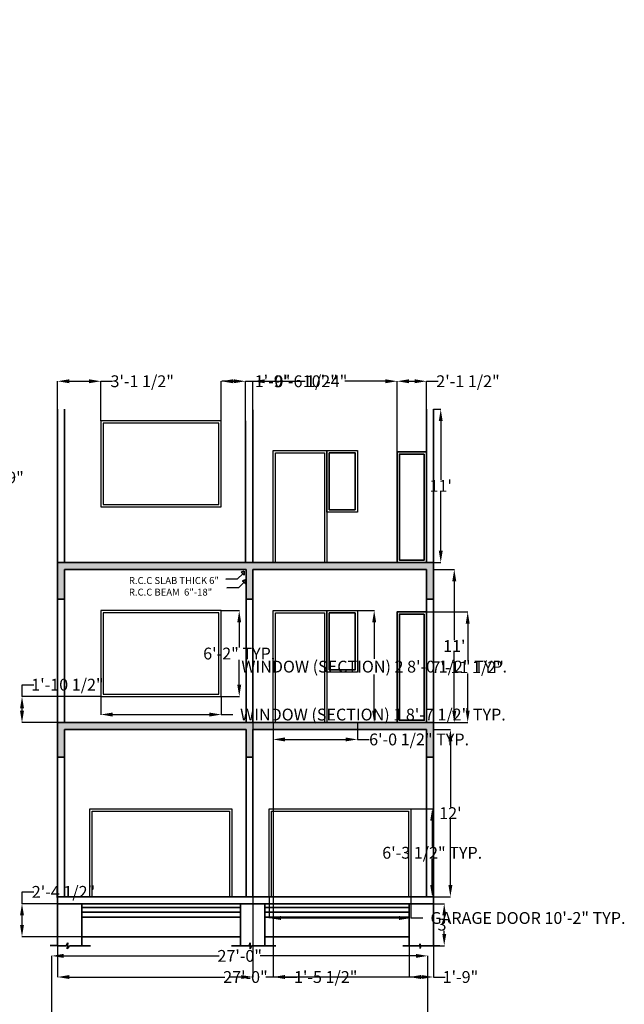
# Model space of a CAD drawing. Units: inches. Extents: x 41 to 5965, y 7 to 3328.
# Tile 6 of 6: x 5444 to 5965, y 2424 to 3272. Entities that reach past the tile are written whole.
import ezdxf

# ---------------------------------------------------------------- set-up
doc = ezdxf.new("R2010")
doc.units = ezdxf.units.IN
doc.header["$MEASUREMENT"] = 0
for name, color, linetype, lineweight in [('A-ANNO-DIMS', 2, 'Continuous', 18), ('A-ANNO-TEXT', 3, 'Continuous', 18), ('A-ELEV', 7, 'Continuous', 25), ('A-SECT', 7, 'Continuous', 35), ('A-SECT-PATT', 8, 'Continuous', 13)]:
    doc.layers.add(name, color=color, linetype=linetype, lineweight=lineweight)
doc.styles.get("Standard").update_dxf_attribs({"font": 'arial.ttf'})
doc.dimstyles.get("Standard").update_dxf_attribs({"dimtxt": 10.18, "dimasz": 10.18, "dimexe": 0.18, "dimexo": 0.0625, "dimgap": 0.09, "dimtad": 0, "dimtih": 1, "dimtoh": 1, "dimdec": 0, "dimzin": 0, "dimdsep": 46, "dimlunit": 3, "dimtxsty": 'Standard', "dimcen": 0.09, "dimadec": 0, "dimazin": 0, "dimtfac": 1, "dimtdec": 0, "dimtofl": 0, "dimtmove": 0, "dimatfit": 3, "dimfxl": 1, "dimtolj": 1, "dimtzin": 0, "dimarcsym": 0})

# ---------------------------------------------------------------- blocks, each defined once
blk = doc.blocks.new('*D9')
at = {"layer": 'A-ANNO-DIMS', "color": 0, "lineweight": -2, "transparency": 16777216}
for p, q in [((5800.43, 2510.77), (5809.93, 2510.77)), ((5809.75, 2500.59), (5809.75, 2497.96)), ((5809.75, 2484.76), (5809.75, 2487.38)), ((5800.43, 2474.58), (5809.93, 2474.58))]:
    blk.add_line(p, q, dxfattribs=at)
at = {"layer": 'A-ANNO-DIMS', "color": 0, "transparency": 16777216}
for points in [[(5808.06, 2500.59), (5811.45, 2500.59), (5809.75, 2510.77)], [(5808.06, 2484.76), (5811.45, 2484.76), (5809.75, 2474.58)]]:
    blk.add_solid(points, dxfattribs=at)
at = {"layer": 'Defpoints', "color": 0, "transparency": 16777216}
for p in [(5800.37, 2510.77), (5809.75, 2510.77), (5800.37, 2474.58)]:
    blk.add_point(p, dxfattribs=at)
at = {"layer": 'A-ANNO-DIMS', "color": 0, "transparency": 16777216, "insert": (5809.75, 2492.67), "char_height": 10.18, "attachment_point": 5}
blk.add_mtext("\\A1;3'", dxfattribs=at)
blk = doc.blocks.new('*D10')
at = {"layer": 'A-ANNO-DIMS', "color": 0, "lineweight": -2, "transparency": 16777216}
for p, q in [((5800.52, 2660.77), (5815.24, 2660.77)), ((5815.06, 2650.59), (5815.06, 2593.97)), ((5815.06, 2526.95), (5815.06, 2583.57)), ((5800.52, 2516.77), (5815.24, 2516.77))]:
    blk.add_line(p, q, dxfattribs=at)
at = {"layer": 'A-ANNO-DIMS', "color": 0, "transparency": 16777216}
for points in [[(5813.37, 2650.59), (5816.76, 2650.59), (5815.06, 2660.77)], [(5813.37, 2526.95), (5816.76, 2526.95), (5815.06, 2516.77)]]:
    blk.add_solid(points, dxfattribs=at)
at = {"layer": 'Defpoints', "color": 0, "transparency": 16777216}
for p in [(5800.46, 2660.77), (5815.06, 2660.77), (5800.46, 2516.77)]:
    blk.add_point(p, dxfattribs=at)
at = {"layer": 'A-ANNO-DIMS', "color": 0, "transparency": 16777216, "insert": (5815.06, 2588.77), "char_height": 10.18, "attachment_point": 5}
blk.add_mtext("\\A1;12'", dxfattribs=at)
blk = doc.blocks.new('*D11')
at = {"layer": 'A-ANNO-DIMS', "color": 0, "lineweight": -2, "transparency": 16777216}
for p, q in [((5800.52, 2798.77), (5818.58, 2798.77)), ((5818.4, 2788.59), (5818.4, 2737.97)), ((5818.4, 2676.95), (5818.4, 2727.57)), ((5800.52, 2666.77), (5818.58, 2666.77))]:
    blk.add_line(p, q, dxfattribs=at)
at = {"layer": 'A-ANNO-DIMS', "color": 0, "transparency": 16777216}
for points in [[(5816.7, 2788.59), (5820.1, 2788.59), (5818.4, 2798.77)], [(5816.7, 2676.95), (5820.1, 2676.95), (5818.4, 2666.77)]]:
    blk.add_solid(points, dxfattribs=at)
at = {"layer": 'Defpoints', "color": 0, "transparency": 16777216}
for p in [(5800.46, 2798.77), (5818.4, 2798.77), (5800.46, 2666.77)]:
    blk.add_point(p, dxfattribs=at)
at = {"layer": 'A-ANNO-DIMS', "color": 0, "transparency": 16777216, "insert": (5818.4, 2732.77), "char_height": 10.18, "attachment_point": 5}
blk.add_mtext("\\A1;11'", dxfattribs=at)
blk = doc.blocks.new('*D12')
at = {"layer": 'A-ANNO-DIMS', "color": 0, "lineweight": -2, "transparency": 16777216}
for p, q in [((5800.52, 2936.77), (5806.9, 2936.77)), ((5806.72, 2926.59), (5806.72, 2875.97)), ((5806.72, 2814.95), (5806.72, 2865.57)), ((5800.52, 2804.77), (5806.9, 2804.77))]:
    blk.add_line(p, q, dxfattribs=at)
at = {"layer": 'A-ANNO-DIMS', "color": 0, "transparency": 16777216}
for points in [[(5805.03, 2926.59), (5808.42, 2926.59), (5806.72, 2936.77)], [(5805.03, 2814.95), (5808.42, 2814.95), (5806.72, 2804.77)]]:
    blk.add_solid(points, dxfattribs=at)
at = {"layer": 'Defpoints', "color": 0, "transparency": 16777216}
for p in [(5800.46, 2936.77), (5806.72, 2936.77), (5800.46, 2804.77)]:
    blk.add_point(p, dxfattribs=at)
at = {"layer": 'A-ANNO-DIMS', "color": 0, "transparency": 16777216, "insert": (5806.72, 2870.77), "char_height": 10.18, "attachment_point": 5}
blk.add_mtext("\\A1;11'", dxfattribs=at)
blk = doc.blocks.new('WIN-SEC-1')
for p, q in [((0, 74.01), (0, 0)), ((103.71, 74.01), (0, 74.01)), ((101.71, 72.01), (2, 72.01)), ((2, 72.01), (2, 2)), ((101.71, 2), (101.71, 72.01)), ((103.71, 0), (103.71, 74.01)), ((2, 2), (101.71, 2)), ((0, 0), (103.71, 0))]:
    blk.add_line(p, q)
blk = doc.blocks.new('WIN-SEC-2')
for p, q in [((0, 0), (0, 96.53)), ((0, 96.53), (46.42, 96.53)), ((2, 94.53), (44.42, 94.53)), ((2, 0), (2, 94.53)), ((44.42, 94.53), (44.42, 0)), ((46.42, 96.53), (46.42, 0))]:
    blk.add_line(p, q)
blk.add_lwpolyline([(46.42, 96.53), (46.42, 96.53), (72.68, 96.53), (72.68, 96.53), (72.68, 43.37), (72.68, 43.37), (46.42, 43.37), (46.42, 43.37)], close=True)
blk = doc.blocks.new('GARAGE-DOOR-ELEV')
for p, q in [((0, 75.7), (122.23, 75.7)), ((0, 0), (0, 75.7)), ((2, 0), (2, 73.7)), ((2, 73.7), (120.23, 73.7)), ((120.23, 73.7), (120.23, 0)), ((122.23, 75.7), (122.23, 0))]:
    blk.add_line(p, q)
blk = doc.blocks.new('*D26')
at = {"layer": 'A-ANNO-DIMS', "color": 0, "lineweight": -2, "transparency": 16777216}
for p, q in [((5513.8, 2689.23), (5513.8, 2673.55)), ((5617.51, 2689.23), (5617.51, 2673.55)), ((5523.98, 2673.73), (5607.33, 2673.73)), ((5617.51, 2673.73), (5627.69, 2673.73))]:
    blk.add_line(p, q, dxfattribs=at)
at = {"layer": 'A-ANNO-DIMS', "color": 0, "transparency": 16777216}
for points in [[(5523.98, 2675.43), (5523.98, 2672.03), (5513.8, 2673.73)], [(5607.33, 2675.43), (5607.33, 2672.03), (5617.51, 2673.73)]]:
    blk.add_solid(points, dxfattribs=at)
at = {"layer": 'Defpoints', "color": 0, "transparency": 16777216}
for p in [(5513.8, 2689.29), (5617.51, 2689.29), (5617.51, 2673.73)]:
    blk.add_point(p, dxfattribs=at)
at = {"layer": 'A-ANNO-DIMS', "color": 0, "transparency": 16777216, "insert": (5748.3, 2673.73), "char_height": 10.18, "attachment_point": 5}
blk.add_mtext('\\A1;WINDOW (SECTION) 1 8\'-7 1/2" TYP.', dxfattribs=at)
blk = doc.blocks.new('*D27')
at = {"layer": 'A-ANNO-DIMS', "color": 0, "lineweight": -2, "transparency": 16777216}
for p, q in [((5617.57, 2763.3), (5633.25, 2763.3)), ((5633.07, 2753.12), (5633.07, 2731.58)), ((5633.07, 2699.47), (5633.07, 2721.01)), ((5617.57, 2689.29), (5633.25, 2689.29))]:
    blk.add_line(p, q, dxfattribs=at)
at = {"layer": 'A-ANNO-DIMS', "color": 0, "transparency": 16777216}
for points in [[(5631.37, 2753.12), (5634.76, 2753.12), (5633.07, 2763.3)], [(5631.37, 2699.47), (5634.76, 2699.47), (5633.07, 2689.29)]]:
    blk.add_solid(points, dxfattribs=at)
at = {"layer": 'Defpoints', "color": 0, "transparency": 16777216}
for p in [(5617.51, 2763.3), (5633.07, 2763.3), (5617.51, 2689.29)]:
    blk.add_point(p, dxfattribs=at)
at = {"layer": 'A-ANNO-DIMS', "color": 0, "transparency": 16777216, "insert": (5633.07, 2726.29), "char_height": 10.18, "attachment_point": 5}
blk.add_mtext('\\A1;6\'-2" TYP.', dxfattribs=at)
blk = doc.blocks.new('*D28')
at = {"layer": 'A-ANNO-DIMS', "color": 0, "lineweight": -2, "transparency": 16777216}
for p, q in [((5734.95, 2763.3), (5749.55, 2763.3)), ((5749.37, 2753.12), (5749.37, 2721.8)), ((5749.37, 2676.95), (5749.37, 2708.27)), ((5734.95, 2666.77), (5749.55, 2666.77))]:
    blk.add_line(p, q, dxfattribs=at)
at = {"layer": 'A-ANNO-DIMS', "color": 0, "transparency": 16777216}
for points in [[(5747.67, 2753.12), (5751.07, 2753.12), (5749.37, 2763.3)], [(5747.67, 2676.95), (5751.07, 2676.95), (5749.37, 2666.77)]]:
    blk.add_solid(points, dxfattribs=at)
at = {"layer": 'Defpoints', "color": 0, "transparency": 16777216}
for p in [(5734.89, 2763.3), (5749.37, 2763.3), (5734.89, 2666.77)]:
    blk.add_point(p, dxfattribs=at)
at = {"layer": 'A-ANNO-DIMS', "color": 0, "transparency": 16777216, "insert": (5749.37, 2715.03), "char_height": 10.18, "attachment_point": 5}
blk.add_mtext('\\A1;WINDOW (SECTION) 2 8\'-0 1/2" TYP.', dxfattribs=at)
blk = doc.blocks.new('*D29')
at = {"layer": 'A-ANNO-DIMS', "color": 0, "lineweight": -2, "transparency": 16777216}
for p, q in [((5662.21, 2666.7), (5662.21, 2652.11)), ((5734.89, 2666.7), (5734.89, 2652.11)), ((5672.39, 2652.29), (5724.71, 2652.29)), ((5734.89, 2652.29), (5745.07, 2652.29))]:
    blk.add_line(p, q, dxfattribs=at)
at = {"layer": 'A-ANNO-DIMS', "color": 0, "transparency": 16777216}
for points in [[(5672.39, 2653.98), (5672.39, 2650.59), (5662.21, 2652.29)], [(5724.71, 2653.98), (5724.71, 2650.59), (5734.89, 2652.29)]]:
    blk.add_solid(points, dxfattribs=at)
at = {"layer": 'Defpoints', "color": 0, "transparency": 16777216}
for p in [(5662.21, 2666.77), (5734.89, 2666.77), (5734.89, 2652.29)]:
    blk.add_point(p, dxfattribs=at)
at = {"layer": 'A-ANNO-DIMS', "color": 0, "transparency": 16777216, "insert": (5788.08, 2652.29), "char_height": 10.18, "attachment_point": 5}
blk.add_mtext('\\A1;6\'-0 1/2" TYP.', dxfattribs=at)
blk = doc.blocks.new('*D30')
at = {"layer": 'A-ANNO-DIMS', "color": 0, "lineweight": -2, "transparency": 16777216}
for p, q in [((5658.8, 2516.7), (5658.8, 2498.25)), ((5781.03, 2516.7), (5781.03, 2498.25)), ((5668.98, 2498.43), (5770.85, 2498.43)), ((5781.03, 2498.43), (5791.21, 2498.43))]:
    blk.add_line(p, q, dxfattribs=at)
at = {"layer": 'A-ANNO-DIMS', "color": 0, "transparency": 16777216}
for points in [[(5668.98, 2500.13), (5668.98, 2496.74), (5658.8, 2498.43)], [(5770.85, 2500.13), (5770.85, 2496.74), (5781.03, 2498.43)]]:
    blk.add_solid(points, dxfattribs=at)
at = {"layer": 'Defpoints', "color": 0, "transparency": 16777216}
for p in [(5658.8, 2516.77), (5781.03, 2516.77), (5781.03, 2498.43)]:
    blk.add_point(p, dxfattribs=at)
at = {"layer": 'A-ANNO-DIMS', "color": 0, "transparency": 16777216, "insert": (5881.91, 2498.43), "char_height": 10.18, "attachment_point": 5}
blk.add_mtext('\\A1;GARAGE DOOR 10\'-2" TYP.', dxfattribs=at)
blk = doc.blocks.new('*D31')
at = {"layer": 'A-ANNO-DIMS', "color": 0, "lineweight": -2, "transparency": 16777216}
for p, q in [((5781.1, 2592.47), (5799.55, 2592.47)), ((5799.37, 2582.29), (5799.37, 2559.98)), ((5799.37, 2526.95), (5799.37, 2549.26)), ((5781.1, 2516.77), (5799.55, 2516.77))]:
    blk.add_line(p, q, dxfattribs=at)
at = {"layer": 'A-ANNO-DIMS', "color": 0, "transparency": 16777216}
for points in [[(5797.67, 2582.29), (5801.06, 2582.29), (5799.37, 2592.47)], [(5797.67, 2526.95), (5801.06, 2526.95), (5799.37, 2516.77)]]:
    blk.add_solid(points, dxfattribs=at)
at = {"layer": 'Defpoints', "color": 0, "transparency": 16777216}
for p in [(5781.03, 2592.47), (5799.37, 2592.47), (5781.03, 2516.77)]:
    blk.add_point(p, dxfattribs=at)
at = {"layer": 'A-ANNO-DIMS', "color": 0, "transparency": 16777216, "insert": (5799.37, 2554.62), "char_height": 10.18, "attachment_point": 5}
blk.add_mtext('\\A1;6\'-3 1/2" TYP.', dxfattribs=at)
blk = doc.blocks.new('*D49')
at = {"layer": 'A-ANNO-DIMS', "color": 0, "lineweight": -2, "transparency": 16777216}
for p, q in [((5471.49, 2414.58), (5471.49, 2465.95)), ((5481.67, 2465.77), (5615.83, 2465.77)), ((5785.31, 2465.77), (5651.16, 2465.77)), ((5795.49, 2414.58), (5795.49, 2465.95))]:
    blk.add_line(p, q, dxfattribs=at)
at = {"layer": 'A-ANNO-DIMS', "color": 0, "transparency": 16777216}
for points in [[(5481.67, 2467.47), (5481.67, 2464.07), (5471.49, 2465.77)], [(5785.31, 2467.47), (5785.31, 2464.07), (5795.49, 2465.77)]]:
    blk.add_solid(points, dxfattribs=at)
at = {"layer": 'Defpoints', "color": 0, "transparency": 16777216}
for p in [(5795.49, 2465.77), (5471.49, 2414.52), (5795.49, 2414.52)]:
    blk.add_point(p, dxfattribs=at)
at = {"layer": 'A-ANNO-DIMS', "color": 0, "transparency": 16777216, "insert": (5633.49, 2465.77), "char_height": 10.18, "attachment_point": 5}
blk.add_mtext('\\A1;27\'-0"', dxfattribs=at)
blk = doc.blocks.new('*D64')
at = {"layer": 'A-ANNO-DIMS', "color": 0, "lineweight": -2, "transparency": 16777216}
for p, q in [((5387.78, 3272.46), (5428.4, 3272.46)), ((5428.22, 3262.28), (5428.22, 2883.29)), ((5428.22, 2493.72), (5428.22, 2872.71)), ((5387.78, 2483.54), (5428.4, 2483.54))]:
    blk.add_line(p, q, dxfattribs=at)
at = {"layer": 'A-ANNO-DIMS', "color": 0, "transparency": 16777216}
for points in [[(5426.52, 3262.28), (5429.92, 3262.28), (5428.22, 3272.46)], [(5426.52, 2493.72), (5429.92, 2493.72), (5428.22, 2483.54)]]:
    blk.add_solid(points, dxfattribs=at)
at = {"layer": 'Defpoints', "color": 0, "transparency": 16777216}
for p in [(5387.72, 3272.46), (5428.22, 3272.46), (5387.72, 2483.54)]:
    blk.add_point(p, dxfattribs=at)
at = {"layer": 'A-ANNO-DIMS', "color": 0, "transparency": 16777216, "insert": (5428.22, 2878), "char_height": 10.18, "attachment_point": 5}
blk.add_mtext('\\A1;65\'-9"', dxfattribs=at)
blk = doc.blocks.new('*D79')
at = {"layer": 'A-ANNO-DIMS', "color": 0, "lineweight": -2, "transparency": 16777216}
for p, q in [((5476.46, 2936.83), (5476.46, 2961.1)), ((5513.8, 2926.75), (5513.8, 2961.1)), ((5486.64, 2960.92), (5503.62, 2960.92)), ((5513.8, 2960.92), (5523.98, 2960.92))]:
    blk.add_line(p, q, dxfattribs=at)
at = {"layer": 'A-ANNO-DIMS', "color": 0, "transparency": 16777216}
for points in [[(5486.64, 2962.61), (5486.64, 2959.22), (5476.46, 2960.92)], [(5503.62, 2962.61), (5503.62, 2959.22), (5513.8, 2960.92)]]:
    blk.add_solid(points, dxfattribs=at)
at = {"layer": 'Defpoints', "color": 0, "transparency": 16777216}
for p in [(5513.8, 2960.92), (5476.46, 2936.77), (5513.8, 2926.68)]:
    blk.add_point(p, dxfattribs=at)
at = {"layer": 'A-ANNO-DIMS', "color": 0, "transparency": 16777216, "insert": (5549.45, 2960.92), "char_height": 10.18, "attachment_point": 5}
blk.add_mtext('\\A1;3\'-1 1/2"', dxfattribs=at)
blk = doc.blocks.new('*D80')
at = {"layer": 'A-ANNO-DIMS', "color": 0, "lineweight": -2, "transparency": 16777216}
for p, q in [((5617.51, 2926.75), (5617.51, 2961.1)), ((5638.46, 2926.75), (5638.46, 2961.1)), ((5627.69, 2960.92), (5628.28, 2960.92)), ((5638.46, 2960.92), (5648.64, 2960.92))]:
    blk.add_line(p, q, dxfattribs=at)
at = {"layer": 'A-ANNO-DIMS', "color": 0, "transparency": 16777216}
for points in [[(5627.69, 2962.61), (5627.69, 2959.22), (5617.51, 2960.92)], [(5628.28, 2962.61), (5628.28, 2959.22), (5638.46, 2960.92)]]:
    blk.add_solid(points, dxfattribs=at)
at = {"layer": 'Defpoints', "color": 0, "transparency": 16777216}
for p in [(5638.46, 2960.92), (5617.51, 2926.68), (5638.46, 2926.68)]:
    blk.add_point(p, dxfattribs=at)
at = {"layer": 'A-ANNO-DIMS', "color": 0, "transparency": 16777216, "insert": (5661.78, 2960.92), "char_height": 10.18, "attachment_point": 5}
blk.add_mtext('\\A1;1\'-9"', dxfattribs=at)
blk = doc.blocks.new('*D81')
at = {"layer": 'A-ANNO-DIMS', "color": 0, "lineweight": -2, "transparency": 16777216}
for p, q in [((5638.46, 2926.75), (5638.46, 2961.1)), ((5644.92, 2936.46), (5644.92, 2961.1)), ((5628.28, 2960.92), (5618.1, 2960.92)), ((5655.1, 2960.92), (5665.28, 2960.92))]:
    blk.add_line(p, q, dxfattribs=at)
at = {"layer": 'A-ANNO-DIMS', "color": 0, "transparency": 16777216}
for points in [[(5628.28, 2962.61), (5628.28, 2959.22), (5638.46, 2960.92)], [(5655.1, 2962.61), (5655.1, 2959.22), (5644.92, 2960.92)]]:
    blk.add_solid(points, dxfattribs=at)
at = {"layer": 'Defpoints', "color": 0, "transparency": 16777216}
for p in [(5644.92, 2960.92), (5644.92, 2936.4), (5638.46, 2926.68)]:
    blk.add_point(p, dxfattribs=at)
at = {"layer": 'A-ANNO-DIMS', "color": 0, "transparency": 16777216, "insert": (5690.76, 2960.92), "char_height": 10.18, "attachment_point": 5}
blk.add_mtext('\\A1;0\'-6 1/2"', dxfattribs=at)
blk = doc.blocks.new('*D82')
at = {"layer": 'A-ANNO-DIMS', "color": 0, "lineweight": -2, "transparency": 16777216}
for p, q in [((5644.92, 2936.46), (5644.92, 2961.1)), ((5769.1, 2900.3), (5769.1, 2961.1)), ((5655.1, 2960.92), (5689.92, 2960.92)), ((5758.92, 2960.92), (5724.11, 2960.92))]:
    blk.add_line(p, q, dxfattribs=at)
at = {"layer": 'A-ANNO-DIMS', "color": 0, "transparency": 16777216}
for points in [[(5655.1, 2962.61), (5655.1, 2959.22), (5644.92, 2960.92)], [(5758.92, 2962.61), (5758.92, 2959.22), (5769.1, 2960.92)]]:
    blk.add_solid(points, dxfattribs=at)
at = {"layer": 'Defpoints', "color": 0, "transparency": 16777216}
for p in [(5769.1, 2960.92), (5644.92, 2936.4), (5769.1, 2900.23)]:
    blk.add_point(p, dxfattribs=at)
at = {"layer": 'A-ANNO-DIMS', "color": 0, "transparency": 16777216, "insert": (5707.01, 2960.92), "char_height": 10.18, "attachment_point": 5}
blk.add_mtext('\\A1;10\'-4"', dxfattribs=at)
blk = doc.blocks.new('*D83')
at = {"layer": 'A-ANNO-DIMS', "color": 0, "lineweight": -2, "transparency": 16777216}
for p, q in [((5769.1, 2900.3), (5769.1, 2961.1)), ((5794.46, 2900.3), (5794.46, 2961.1)), ((5779.28, 2960.92), (5784.28, 2960.92)), ((5794.46, 2960.92), (5804.64, 2960.92))]:
    blk.add_line(p, q, dxfattribs=at)
at = {"layer": 'A-ANNO-DIMS', "color": 0, "transparency": 16777216}
for points in [[(5779.28, 2962.61), (5779.28, 2959.22), (5769.1, 2960.92)], [(5784.28, 2962.61), (5784.28, 2959.22), (5794.46, 2960.92)]]:
    blk.add_solid(points, dxfattribs=at)
at = {"layer": 'Defpoints', "color": 0, "transparency": 16777216}
for p in [(5794.46, 2960.92), (5769.1, 2900.23), (5794.46, 2900.23)]:
    blk.add_point(p, dxfattribs=at)
at = {"layer": 'A-ANNO-DIMS', "color": 0, "transparency": 16777216, "insert": (5830.2, 2960.92), "char_height": 10.18, "attachment_point": 5}
blk.add_mtext('\\A1;2\'-1 1/2"', dxfattribs=at)
blk = doc.blocks.new('*D84')
at = {"layer": 'A-ANNO-DIMS', "color": 0, "lineweight": -2, "transparency": 16777216}
for p, q in [((5445.86, 2689.29), (5445.86, 2699.47)), ((5445.86, 2699.47), (5456.04, 2699.47)), ((5513.73, 2689.29), (5445.68, 2689.29)), ((5445.86, 2676.95), (5445.86, 2679.11)), ((5482.39, 2666.77), (5445.68, 2666.77))]:
    blk.add_line(p, q, dxfattribs=at)
at = {"layer": 'A-ANNO-DIMS', "color": 0, "transparency": 16777216}
for points in [[(5444.17, 2679.11), (5447.56, 2679.11), (5445.86, 2689.29)], [(5444.17, 2676.95), (5447.56, 2676.95), (5445.86, 2666.77)]]:
    blk.add_solid(points, dxfattribs=at)
at = {"layer": 'Defpoints', "color": 0, "transparency": 16777216}
for p in [(5445.86, 2689.29), (5513.8, 2689.29), (5482.46, 2666.77)]:
    blk.add_point(p, dxfattribs=at)
at = {"layer": 'A-ANNO-DIMS', "color": 0, "transparency": 16777216, "insert": (5485, 2699.47), "char_height": 10.18, "attachment_point": 5}
blk.add_mtext('\\A1;1\'-10 1/2"', dxfattribs=at)
blk = doc.blocks.new('*D85')
at = {"layer": 'A-ANNO-DIMS', "color": 0, "lineweight": -2, "transparency": 16777216}
for p, q in [((5644.92, 2666.7), (5644.92, 2447.4)), ((5662.21, 2666.7), (5662.21, 2447.4)), ((5634.74, 2447.58), (5624.56, 2447.58)), ((5672.39, 2447.58), (5682.57, 2447.58))]:
    blk.add_line(p, q, dxfattribs=at)
at = {"layer": 'A-ANNO-DIMS', "color": 0, "transparency": 16777216}
for points in [[(5634.74, 2449.28), (5634.74, 2445.88), (5644.92, 2447.58)], [(5672.39, 2449.28), (5672.39, 2445.88), (5662.21, 2447.58)]]:
    blk.add_solid(points, dxfattribs=at)
at = {"layer": 'Defpoints', "color": 0, "transparency": 16777216}
for p in [(5644.92, 2666.77), (5662.21, 2666.77), (5662.21, 2447.58)]:
    blk.add_point(p, dxfattribs=at)
at = {"layer": 'A-ANNO-DIMS', "color": 0, "transparency": 16777216, "insert": (5707.58, 2447.58), "char_height": 10.18, "attachment_point": 5}
blk.add_mtext('\\A1;1\'-5 1/2"', dxfattribs=at)
blk = doc.blocks.new('*D86')
at = {"layer": 'A-ANNO-DIMS', "color": 0, "lineweight": -2, "transparency": 16777216}
for p, q in [((5769.17, 2762.23), (5830.14, 2762.23)), ((5829.96, 2752.05), (5829.96, 2719.85)), ((5829.96, 2676.95), (5829.96, 2709.15)), ((5769.17, 2666.77), (5830.14, 2666.77))]:
    blk.add_line(p, q, dxfattribs=at)
at = {"layer": 'A-ANNO-DIMS', "color": 0, "transparency": 16777216}
for points in [[(5828.27, 2752.05), (5831.66, 2752.05), (5829.96, 2762.23)], [(5828.27, 2676.95), (5831.66, 2676.95), (5829.96, 2666.77)]]:
    blk.add_solid(points, dxfattribs=at)
at = {"layer": 'Defpoints', "color": 0, "transparency": 16777216}
for p in [(5769.1, 2762.23), (5829.96, 2762.23), (5769.1, 2666.77)]:
    blk.add_point(p, dxfattribs=at)
at = {"layer": 'A-ANNO-DIMS', "color": 0, "transparency": 16777216, "insert": (5829.96, 2714.5), "char_height": 10.18, "attachment_point": 5}
blk.add_mtext('\\A1;7\'-11 1/2"', dxfattribs=at)
blk = doc.blocks.new('*D87')
at = {"layer": 'A-ANNO-DIMS', "color": 0, "lineweight": -2, "transparency": 16777216}
for p, q in [((5779.47, 2474.51), (5779.47, 2447.4)), ((5800.37, 2474.51), (5800.37, 2447.4)), ((5789.65, 2447.58), (5790.19, 2447.58)), ((5800.37, 2447.58), (5810.55, 2447.58))]:
    blk.add_line(p, q, dxfattribs=at)
at = {"layer": 'A-ANNO-DIMS', "color": 0, "transparency": 16777216}
for points in [[(5789.65, 2449.28), (5789.65, 2445.88), (5779.47, 2447.58)], [(5790.19, 2449.28), (5790.19, 2445.88), (5800.37, 2447.58)]]:
    blk.add_solid(points, dxfattribs=at)
at = {"layer": 'Defpoints', "color": 0, "transparency": 16777216}
for p in [(5779.47, 2474.58), (5800.37, 2474.58), (5800.37, 2447.58)]:
    blk.add_point(p, dxfattribs=at)
at = {"layer": 'A-ANNO-DIMS', "color": 0, "transparency": 16777216, "insert": (5823.69, 2447.58), "char_height": 10.18, "attachment_point": 5}
blk.add_mtext('\\A1;1\'-9"', dxfattribs=at)
blk = doc.blocks.new('*D88')
at = {"layer": 'A-ANNO-DIMS', "color": 0, "lineweight": -2, "transparency": 16777216}
for p, q in [((5445.86, 2510.77), (5445.86, 2520.95)), ((5445.86, 2520.95), (5456.04, 2520.95)), ((5497.29, 2510.77), (5445.68, 2510.77)), ((5445.86, 2492.46), (5445.86, 2500.59)), ((5497.29, 2482.28), (5445.68, 2482.28))]:
    blk.add_line(p, q, dxfattribs=at)
at = {"layer": 'A-ANNO-DIMS', "color": 0, "transparency": 16777216}
for points in [[(5444.17, 2500.59), (5447.56, 2500.59), (5445.86, 2510.77)], [(5444.17, 2492.46), (5447.56, 2492.46), (5445.86, 2482.28)]]:
    blk.add_solid(points, dxfattribs=at)
at = {"layer": 'Defpoints', "color": 0, "transparency": 16777216}
for p in [(5445.86, 2510.77), (5497.35, 2510.77), (5497.35, 2482.28)]:
    blk.add_point(p, dxfattribs=at)
at = {"layer": 'A-ANNO-DIMS', "color": 0, "transparency": 16777216, "insert": (5481.61, 2520.95), "char_height": 10.18, "attachment_point": 5}
blk.add_mtext('\\A1;2\'-4 1/2"', dxfattribs=at)
blk = doc.blocks.new('*D89')
at = {"layer": 'A-ANNO-DIMS', "color": 0, "lineweight": -2, "transparency": 16777216}
for p, q in [((5476.46, 2474.51), (5476.46, 2447.4)), ((5800.37, 2474.51), (5800.37, 2447.4)), ((5486.64, 2447.58), (5620.75, 2447.58)), ((5790.19, 2447.58), (5656.07, 2447.58))]:
    blk.add_line(p, q, dxfattribs=at)
at = {"layer": 'A-ANNO-DIMS', "color": 0, "transparency": 16777216}
for points in [[(5486.64, 2449.28), (5486.64, 2445.88), (5476.46, 2447.58)], [(5790.19, 2449.28), (5790.19, 2445.88), (5800.37, 2447.58)]]:
    blk.add_solid(points, dxfattribs=at)
at = {"layer": 'Defpoints', "color": 0, "transparency": 16777216}
for p in [(5476.46, 2474.58), (5800.37, 2474.58), (5800.37, 2447.58)]:
    blk.add_point(p, dxfattribs=at)
at = {"layer": 'A-ANNO-DIMS', "color": 0, "transparency": 16777216, "insert": (5638.41, 2447.58), "char_height": 10.18, "attachment_point": 5}
blk.add_mtext('\\A1;27\'-0"', dxfattribs=at)

msp = doc.modelspace()

# ---------------------------------------------------------------- hatches: boundary and pattern name
at = {"layer": 'A-SECT-PATT'}
h = msp.add_hatch(color=256, dxfattribs=at)
h.dxf.hatch_style = 1
h.paths.add_polyline_path([(5800.46, 2804.77), (5476.46, 2804.77), (5476.46, 2798.77), (5476.46, 2773.22), (5482.46, 2773.22), (5482.46, 2798.77), (5638.92, 2798.77), (5638.92, 2773.22), (5644.92, 2773.22), (5644.92, 2798.77), (5794.46, 2798.77), (5794.46, 2773.22), (5800.46, 2773.22), (5800.46, 2798.77)])
h = msp.add_hatch(color=256, dxfattribs=at)
h.dxf.hatch_style = 1
h.paths.add_polyline_path([(5638.92, 2660.77), (5638.92, 2636.96), (5644.92, 2636.96), (5644.92, 2660.77), (5794.46, 2660.77), (5794.46, 2636.96), (5800.46, 2636.96), (5800.46, 2660.77), (5800.46, 2666.77), (5476.46, 2666.77), (5476.46, 2660.77), (5476.46, 2636.96), (5482.46, 2636.96), (5482.46, 2660.77)])

# ---------------------------------------------------------------- linework, layer by layer
at = {"layer": 'A-SECT'}
for p, q in [((5476.46, 2804.77), (5476.46, 2936.77)), ((5482.46, 2804.77), (5482.46, 2936.77)), ((5644.92, 2804.77), (5644.92, 2936.4)), ((5794.46, 2804.77), (5794.46, 2936.77)), ((5800.46, 2804.77), (5800.46, 2936.77)), ((5638.46, 2804.77), (5638.46, 2926.68)), ((5476.46, 2804.77), (5800.46, 2804.77)), ((5476.46, 2798.77), (5476.46, 2804.77)), ((5800.46, 2798.77), (5800.46, 2804.77)), ((5476.46, 2666.77), (5476.46, 2798.77)), ((5482.46, 2798.77), (5638.92, 2798.77)), ((5482.46, 2666.77), (5482.46, 2798.77)), ((5631.57, 2790.59), (5636.08, 2795.12)), ((5637.3, 2797.29), (5634.79, 2796.41)), ((5636.08, 2795.12), (5634.79, 2796.41)), ((5634.79, 2796.41), (5637.3, 2793.9)), ((5637.3, 2793.9), (5637.3, 2797.29)), ((5638.92, 2666.77), (5638.92, 2798.77)), ((5644.92, 2798.77), (5794.46, 2798.77)), ((5644.92, 2666.77), (5644.92, 2798.77)), ((5794.46, 2798.77), (5794.46, 2666.77)), ((5800.46, 2798.77), (5800.46, 2666.77)), ((5621.39, 2790.25), (5631.57, 2790.59)), ((5622.51, 2782.79), (5632.69, 2783.13)), ((5632.69, 2783.13), (5637.2, 2787.67)), ((5638.43, 2789.83), (5635.91, 2788.95)), ((5637.2, 2787.67), (5635.91, 2788.95)), ((5635.91, 2788.95), (5638.43, 2786.45)), ((5638.43, 2786.45), (5638.43, 2789.83)), ((5476.46, 2773.22), (5482.46, 2773.22)), ((5638.92, 2773.22), (5644.92, 2773.22)), ((5794.46, 2773.22), (5800.46, 2773.22)), ((5800.46, 2666.77), (5476.46, 2666.77)), ((5476.46, 2666.77), (5476.46, 2660.77)), ((5800.46, 2666.77), (5800.46, 2660.77)), ((5476.46, 2516.77), (5476.46, 2660.77)), ((5482.46, 2516.77), (5482.46, 2660.77)), ((5638.92, 2660.77), (5482.46, 2660.77)), ((5638.92, 2516.77), (5638.92, 2660.77)), ((5794.46, 2660.77), (5644.92, 2660.77)), ((5644.92, 2516.77), (5644.92, 2660.77)), ((5794.46, 2516.77), (5794.46, 2660.77)), ((5800.46, 2516.77), (5800.46, 2660.77)), ((5476.46, 2636.96), (5482.46, 2636.96)), ((5638.92, 2636.96), (5644.92, 2636.96)), ((5794.46, 2636.96), (5800.46, 2636.96)), ((5800.46, 2516.77), (5476.46, 2516.77)), ((5476.46, 2516.77), (5476.46, 2510.77)), ((5800.46, 2510.77), (5800.46, 2516.77)), ((5476.46, 2510.77), (5800.46, 2510.77)), ((5476.46, 2510.77), (5476.46, 2474.77)), ((5497.35, 2507.5), (5634.14, 2507.5)), ((5497.35, 2503.4), (5634.14, 2503.4)), ((5655.03, 2507.5), (5779.47, 2507.5)), ((5655.03, 2503.4), (5779.47, 2503.4)), ((5497.35, 2499.05), (5634.14, 2499.05)), ((5655.03, 2499.05), (5779.47, 2499.05)), ((5497.35, 2482.28), (5634.14, 2482.28)), ((5655.03, 2482.28), (5779.47, 2482.28)), ((5476.29, 2474.86), (5470.01, 2474.86)), ((5476.46, 2474.58), (5483.85, 2474.58)), ((5483.85, 2474.58), (5485.34, 2477.16)), ((5485.34, 2477.16), (5484.69, 2471.73)), ((5484.69, 2471.73), (5486.9, 2474.58)), ((5497.35, 2474.58), (5504.98, 2474.58)), ((5634.14, 2474.58), (5626.36, 2474.58)), ((5634.14, 2474.58), (5641.73, 2474.58)), ((5641.73, 2474.58), (5642.46, 2477.06)), ((5642.46, 2477.06), (5642.46, 2471.91)), ((5642.46, 2471.91), (5643.63, 2474.58)), ((5655.03, 2474.58), (5664.64, 2474.58)), ((5779.47, 2474.58), (5774.12, 2474.58)), ((5774.12, 2474.58), (5774.12, 2474.58)), ((5779.47, 2474.58), (5788.34, 2474.58)), ((5788.34, 2474.58), (5788.92, 2476.08)), ((5788.92, 2476.08), (5789.12, 2472.19)), ((5789.12, 2472.19), (5789.65, 2474.58)), ((5800.37, 2474.58), (5805.81, 2474.58))]:
    msp.add_line(p, q, dxfattribs=at)
for points in [[(5710.64, 2899.3), (5732.89, 2899.3), (5732.89, 2850.14), (5710.64, 2850.14)], [(5794.46, 2900.23), (5794.46, 2900.23), (5769.1, 2900.23), (5769.1, 2900.23), (5769.1, 2804.77), (5769.1, 2804.77), (5794.46, 2804.77), (5794.46, 2804.77)], [(5792.46, 2898.23), (5771.1, 2898.23), (5771.1, 2806.77), (5792.46, 2806.77)], [(5710.64, 2761.3), (5732.89, 2761.3), (5732.89, 2712.14), (5710.64, 2712.14)], [(5794.46, 2762.23), (5794.46, 2762.23), (5769.1, 2762.23), (5769.1, 2762.23), (5769.1, 2666.77), (5769.1, 2666.77), (5794.46, 2666.77), (5794.46, 2666.77)], [(5792.46, 2760.23), (5771.1, 2760.23), (5771.1, 2668.77), (5792.46, 2668.77)]]:
    msp.add_lwpolyline(points, close=True, dxfattribs=at)
for points in [[(5483.85, 2474.58), (5476.46, 2474.58), (5476.46, 2474.58), (5476.46, 2510.77), (5476.46, 2510.77), (5497.35, 2510.77), (5497.35, 2510.77), (5497.35, 2474.58), (5497.35, 2474.58), (5486.9, 2474.58)], [(5641.73, 2474.58), (5634.14, 2474.58), (5634.14, 2474.58), (5634.14, 2510.77), (5634.14, 2510.77), (5655.03, 2510.77), (5655.03, 2510.77), (5655.03, 2474.58), (5655.03, 2474.58), (5643.63, 2474.58)], [(5788.34, 2474.58), (5779.47, 2474.58), (5779.47, 2474.58), (5779.47, 2510.77), (5779.47, 2510.77), (5800.37, 2510.77), (5800.37, 2510.77), (5800.37, 2474.58), (5800.37, 2474.58), (5789.65, 2474.58)]]:
    msp.add_lwpolyline(points, dxfattribs=at)

# ---------------------------------------------------------------- block references
at = {"layer": 'A-ELEV'}
for name, p in [('WIN-SEC-1', (5513.8, 2852.67)), ('WIN-SEC-2', (5662.21, 2804.77)), ('WIN-SEC-1', (5513.8, 2689.29)), ('WIN-SEC-2', (5662.21, 2666.77)), ('GARAGE-DOOR-ELEV', (5504.42, 2516.77)), ('GARAGE-DOOR-ELEV', (5658.8, 2516.77))]:
    msp.add_blockref(name, p, dxfattribs=at)

# ---------------------------------------------------------------- texts
at = {"layer": 'A-ANNO-TEXT', "insert": (5537.99, 2792.21), "char_height": 6, "attachment_point": 1}
msp.add_mtext_dynamic_manual_height_columns('R.C.C SLAB THICK 6" \\PR.C.C BEAM  6"-18"', width=104.6667, gutter_width=1, heights=[0], dxfattribs=at)

# ---------------------------------------------------------------- dimensions: what is measured, and where the dimension line sits
at = {"layer": 'A-ANNO-DIMS'}
for base, p1, p2, override, picture, middle in [((5428.22, 3272.46), (5387.72, 2483.54), (5387.72, 3272.46), {"dimdec": 1, "dimlfac": 1, "dimrnd": 0, "dimzin": 1, "dimdsep": 46, "dimlunit": 4, "dimfrac": 2}, '*D64', (5428.22, 2878)), ((5806.72, 2936.77), (5800.46, 2804.77), (5800.46, 2936.77), {"dimclrd": 0, "dimclre": 0, "dimclrt": 0}, '*D12', (5806.72, 2870.77)), ((5818.4, 2798.77), (5800.46, 2666.77), (5800.46, 2798.77), {"dimclrd": 0, "dimclre": 0, "dimclrt": 0}, '*D11', (5818.4, 2732.77)), ((5829.96, 2762.23), (5769.1, 2666.77), (5769.1, 2762.23), {"dimdec": 1, "dimlfac": 1, "dimrnd": 0, "dimzin": 1, "dimdsep": 46, "dimlunit": 4, "dimfrac": 2}, '*D86', (5829.96, 2714.5)), ((5445.86, 2689.29), (5482.46, 2666.77), (5513.8, 2689.29), {"dimdec": 1, "dimlfac": 1, "dimrnd": 0, "dimzin": 1, "dimdsep": 46, "dimlunit": 4, "dimfrac": 2}, '*D84', (5485, 2699.47)), ((5815.06, 2660.77), (5800.46, 2516.77), (5800.46, 2660.77), {"dimclrd": 0, "dimclre": 0, "dimclrt": 0}, '*D10', (5815.06, 2588.77)), ((5445.86, 2510.77), (5497.35, 2482.28), (5497.35, 2510.77), {"dimdec": 1, "dimlfac": 1, "dimrnd": 0, "dimzin": 1, "dimdsep": 46, "dimlunit": 4, "dimfrac": 2}, '*D88', (5481.61, 2520.95)), ((5809.75, 2510.77), (5800.37, 2474.58), (5800.37, 2510.77), {"dimclrd": 0, "dimclre": 0, "dimclrt": 0}, '*D9', (5809.75, 2492.67))]:
    dim = msp.add_linear_dim(base=base, p1=p1, p2=p2, angle=90, dimstyle='Standard', override=override, dxfattribs=at)
    dim.commit()
    dim.dimension.update_dxf_attribs({"geometry": picture, "text_midpoint": middle})
for base, p1, p2, picture, middle in [((5513.8, 2960.92), (5476.46, 2936.77), (5513.8, 2926.68), '*D79', (5549.45, 2960.92)), ((5644.92, 2960.92), (5638.46, 2926.68), (5644.92, 2936.4), '*D81', (5690.76, 2960.92)), ((5794.46, 2960.92), (5769.1, 2900.23), (5794.46, 2900.23), '*D83', (5830.2, 2960.92)), ((5638.4567, 2960.917), (5617.5086, 2926.6827), (5638.4567, 2926.6827), '*D80', (5661.778, 2960.917)), ((5769.1, 2960.92), (5644.92, 2936.4), (5769.1, 2900.23), '*D82', (5707.01, 2960.92)), ((5662.21, 2447.58), (5644.92, 2666.77), (5662.21, 2666.77), '*D85', (5707.58, 2447.58)), ((5795.49, 2465.77), (5471.49, 2414.52), (5795.49, 2414.52), '*D49', (5633.49, 2465.77)), ((5800.37, 2447.58), (5476.46, 2474.58), (5800.37, 2474.58), '*D89', (5638.41, 2447.58)), ((5800.37, 2447.58), (5779.47, 2474.58), (5800.37, 2474.58), '*D87', (5823.69, 2447.58))]:
    dim = msp.add_linear_dim(base=base, p1=p1, p2=p2, dimstyle='Standard', override={"dimdec": 1, "dimlfac": 1, "dimrnd": 0, "dimzin": 1, "dimdsep": 46, "dimlunit": 4, "dimfrac": 2}, dxfattribs=at)
    dim.commit()
    dim.dimension.update_dxf_attribs({"geometry": picture, "text_midpoint": middle})
for base, p1, p2, text, picture, middle in [((5633.07, 2763.3), (5617.51, 2689.29), (5617.51, 2763.3), '<> TYP.', '*D27', (5633.07, 2726.29)), ((5749.37, 2763.3), (5734.89, 2666.77), (5734.89, 2763.3), 'WINDOW (SECTION) 2 <> TYP.', '*D28', (5749.37, 2715.03)), ((5799.37, 2592.47), (5781.03, 2516.77), (5781.03, 2592.47), '<> TYP.', '*D31', (5799.37, 2554.62))]:
    dim = msp.add_linear_dim(base=base, p1=p1, p2=p2, angle=90, text=text, dimstyle='Standard', override={"dimdec": 1, "dimrnd": 0, "dimzin": 1, "dimlunit": 4, "dimfrac": 2}, dxfattribs=at)
    dim.commit()
    dim.dimension.update_dxf_attribs({"geometry": picture, "text_midpoint": middle})
for base, p1, p2, text, picture, middle in [((5617.51, 2673.73), (5513.8, 2689.29), (5617.51, 2689.29), 'WINDOW (SECTION) 1 <> TYP.', '*D26', (5748.3, 2673.73)), ((5734.89, 2652.29), (5662.21, 2666.77), (5734.89, 2666.77), '<> TYP.', '*D29', (5788.08, 2652.29)), ((5781.03, 2498.43), (5658.8, 2516.77), (5781.03, 2516.77), 'GARAGE DOOR <> TYP.', '*D30', (5881.91, 2498.43))]:
    dim = msp.add_linear_dim(base=base, p1=p1, p2=p2, text=text, dimstyle='Standard', override={"dimdec": 1, "dimrnd": 0, "dimzin": 1, "dimlunit": 4, "dimfrac": 2}, dxfattribs=at)
    dim.commit()
    dim.dimension.update_dxf_attribs({"geometry": picture, "text_midpoint": middle})

doc.saveas('drawing.dxf')
